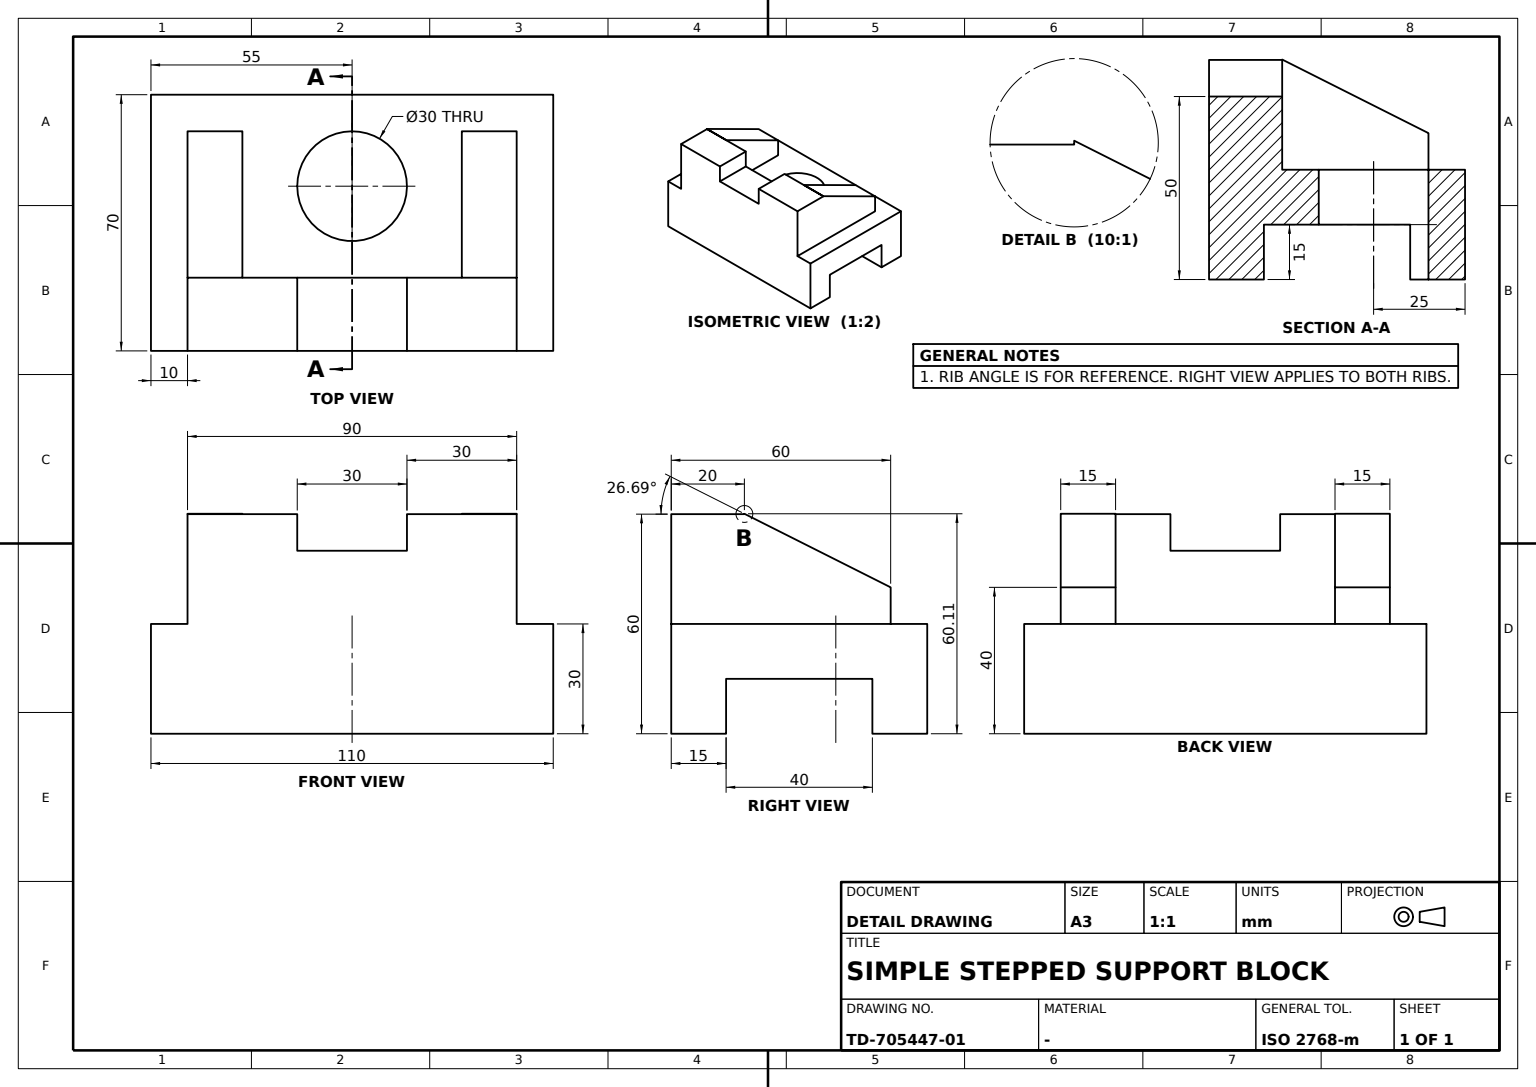
CATIA V5 part; units mm, degrees
sketch "Sketch1" plane through (0, 0, 0) normal (1, 0, 0) x (0, 1, 0)
  line L0 (-20, -22.5) -> (-35, -22.5)
  line L1 (-35, -22.5) -> (-35, 7.5)
  line L2 (-35, 7.5) -> (35, 7.5)
  line L3 (35, 7.5) -> (35, -22.5)
  point P0 (35, -22.5)
  line L4 (35, -22.5) -> (20, -22.5)
  line L5 (20, -22.5) -> (20, -7.5)
  line L6 (20, -7.5) -> (-20, -7.5)
  line L7 (-20, -7.5) -> (-20, -22.5)
  dimension "length L1" = 30
  dimension "length L7" = 15
  dimension "length L2" = 70
  dimension "distance L7 L5" = 40
  constraint horizontal L0 x-axis
  constraint horizontal L2 x-axis
  constraint horizontal L4 x-axis
  constraint horizontal L6 x-axis
  constraint vertical L1 y-axis
  constraint vertical L3 y-axis
  constraint vertical L5 y-axis
  constraint vertical L7 y-axis
  constraint coincidence P0 L0
  constraint symmetry L1 L3 y-axis
  constraint symmetry L2 L6 x-axis
  constraint symmetry L7 L5 y-axis
extrude "Pad1" add sketch "Sketch1" along normal mid plane 110
sketch "Sketch2" plane through (0, -35, 0) normal (0, -1, 0) x (1, 0, 0)
  line L0 (-45, 7.5) -> (45, 7.5)
  line L1 (45, 7.5) -> (45, 37.5)
  line L2 (45, 37.5) -> (15, 37.5)
  line L3 (15, 37.5) -> (15, 27.5)
  line L4 (15, 27.5) -> (-15, 27.5)
  line L5 (-15, 27.5) -> (-15, 37.5)
  point P0 (-15, 37.5)
  line L6 (-15, 37.5) -> (-45, 37.5)
  line L7 (-45, 37.5) -> (-45, 7.5)
  line L8 (-55, 7.5) -> (55, 7.5) construction
  dimension "length L1" = 30
  dimension "distance L5 L3" = 30
  dimension "length L0" = 90
  dimension "length L3" = 10
  constraint horizontal L0 x-axis
  constraint horizontal L2 x-axis
  constraint horizontal L4 x-axis
  constraint horizontal L6 x-axis
  constraint vertical L1 y-axis
  constraint vertical L3 y-axis
  constraint vertical L5 y-axis
  constraint vertical L7 y-axis
  constraint coincidence P0 L2
  constraint coincidence L0 L8
  constraint symmetry L7 L1 y-axis
  constraint symmetry L5 L3 y-axis
extrude "Pad2" add sketch "Sketch2" against normal blind 20
sketch "Sketch3" plane through (45, 0, 0) normal (1, 0, 0) x (0, 1, 0)
  line L0 (-15, 37.6058) -> (25, 17.5)
  line L1 (25, 17.5) -> (25, 7.5)
  line L2 (25, 7.5) -> (-15, 7.5)
  line L3 (-15, 7.5) -> (-15, 37.6058)
  line L4 (-15, 7.5) -> (-15, 37.5) construction
  line L5 (35, 7.5) -> (-35, 7.5) construction
  dimension "length L1" = 10
  dimension "length L2" = 40
  dimension "length L0" = 44.7688
  constraint vertical L1 y-axis
  constraint vertical L3 y-axis
  constraint horizontal L2 x-axis
  constraint coincidence L3 L4
  constraint coincidence L2 L5
extrude "Pad3" add sketch "Sketch3" against normal blind 15
mirror "Mirror1" about plane through (0, 0, 0) normal (1, 0, 0) of "Pad3"
sketch "Sketch4" plane through (-1.4686, 8.5239, 7.5) normal (0, 0, 1) x (1, 0, 0)
  point P0 (1.4686, 1.4761)
  line L0 (-53.5314, 26.4761) -> (56.4686, 26.4761) construction
  line L1 (16.4686, -43.5239) -> (16.4686, -23.5239) construction
  dimension "distance P0 L0" = 25
  dimension "distance P0 L1" = 15
hole "Hole1" at (0, 10, 7.5) direction (0, 0, -1) diameter 30 end through all
